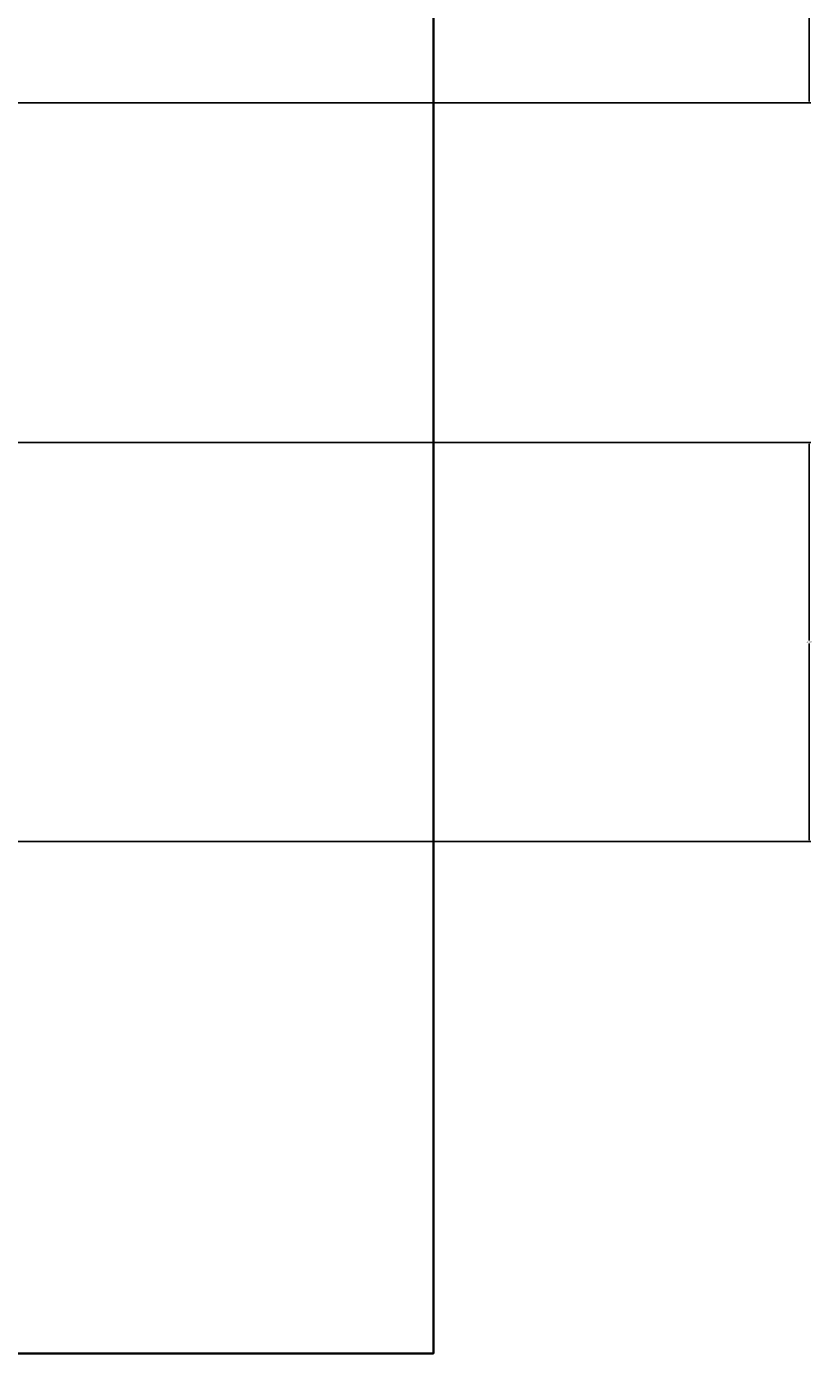
# Model space of a CAD drawing. Units: feet. Extents: x 2100 to 2836, y 2433 to 3396.
# Tile 5 of 12: x 2743 to 2836, y 2477 to 2634. Entities that reach past the tile are written whole.
import ezdxf

# ---------------------------------------------------------------- set-up
doc = ezdxf.new("R2010")
doc.units = ezdxf.units.FT
doc.layers.add('A-ANNO-DIMS', color=2, linetype='Continuous', lineweight=18)
doc.layers.add('A-ANNO-TTLB', color=7, linetype='Continuous', lineweight=35)
doc.styles.get("Standard").update_dxf_attribs({"font": 'arial.ttf'})
doc.dimstyles.get("Standard").update_dxf_attribs({"dimtxt": 0.18, "dimasz": 0.18, "dimexe": 0.18, "dimexo": 0.0625, "dimgap": 0.09, "dimtad": 0, "dimtih": 1, "dimtoh": 1, "dimdec": 4, "dimzin": 0, "dimdsep": 46, "dimtxsty": 'Standard', "dimcen": 0.09, "dimadec": 0, "dimazin": 0, "dimtfac": 1, "dimtdec": 4, "dimtofl": 0, "dimtmove": 0, "dimatfit": 3, "dimfxl": 1, "dimtolj": 1, "dimtzin": 0, "dimarcsym": 0})

# ---------------------------------------------------------------- blocks, each defined once
blk = doc.blocks.new('*D56')
at = {"layer": 'A-ANNO-DIMS', "color": 0, "lineweight": -2, "transparency": 16777216}
for p, q in [((2741.01, 2584.8), (2835.49, 2584.8)), ((2835.31, 2584.62), (2835.31, 2561.46)), ((2835.31, 2537.94), (2835.31, 2561.1)), ((2741.01, 2537.76), (2835.49, 2537.76))]:
    blk.add_line(p, q, dxfattribs=at)
at = {"layer": 'A-ANNO-DIMS', "color": 0, "transparency": 16777216}
for points in [[(2835.28, 2584.62), (2835.34, 2584.62), (2835.31, 2584.8)], [(2835.28, 2537.94), (2835.34, 2537.94), (2835.31, 2537.76)]]:
    blk.add_solid(points, dxfattribs=at)
at = {"layer": 'Defpoints', "color": 0, "transparency": 16777216}
for p in [(2740.95, 2584.8), (2835.31, 2584.8), (2740.95, 2537.76)]:
    blk.add_point(p, dxfattribs=at)
at = {"layer": 'A-ANNO-DIMS', "color": 0, "transparency": 16777216, "insert": (2835.31, 2561.28), "char_height": 0.18, "attachment_point": 5}
blk.add_mtext('\\A1;47.05', dxfattribs=at)
blk = doc.blocks.new('*D57')
at = {"layer": 'A-ANNO-DIMS', "color": 0, "lineweight": -2, "transparency": 16777216}
for p, q in [((2741.01, 2662.65), (2835.49, 2662.65)), ((2835.31, 2662.47), (2835.31, 2643.91)), ((2835.31, 2624.98), (2835.31, 2643.54)), ((2741.01, 2624.8), (2835.49, 2624.8))]:
    blk.add_line(p, q, dxfattribs=at)
at = {"layer": 'A-ANNO-DIMS', "color": 0, "transparency": 16777216}
for points in [[(2835.28, 2662.47), (2835.34, 2662.47), (2835.31, 2662.65)], [(2835.28, 2624.98), (2835.34, 2624.98), (2835.31, 2624.8)]]:
    blk.add_solid(points, dxfattribs=at)
at = {"layer": 'Defpoints', "color": 0, "transparency": 16777216}
for p in [(2740.95, 2662.65), (2835.31, 2662.65), (2740.95, 2624.8)]:
    blk.add_point(p, dxfattribs=at)
at = {"layer": 'A-ANNO-DIMS', "color": 0, "transparency": 16777216, "insert": (2835.31, 2643.73), "char_height": 0.18, "attachment_point": 5}
blk.add_mtext('\\A1;37.845', dxfattribs=at)

msp = doc.modelspace()

# ---------------------------------------------------------------- linework, layer by layer
at = {"layer": 'A-ANNO-TTLB'}
msp.add_lwpolyline([(2144.0848, 3351.6245), (2791.0561, 3351.6245), (2791.0561, 2477.4373), (2144.0848, 2477.4373)], close=True, dxfattribs=at)

# ---------------------------------------------------------------- dimensions: what is measured, and where the dimension line sits
at = {"layer": 'A-ANNO-DIMS'}
for base, p1, p2, override, picture, middle in [((2835.3061, 2662.6479), (2740.9476, 2624.8031), (2740.9476, 2662.6479), {"dimdec": 3, "dimlfac": 1, "dimrnd": 0, "dimzin": 0, "dimdsep": 46, "dimlunit": 2}, '*D57', (2835.3061, 2643.7255)), ((2835.3061, 2584.8031), (2740.9476, 2537.755), (2740.9476, 2584.8031), {"dimdec": 2, "dimlfac": 1, "dimrnd": 0, "dimzin": 0, "dimdsep": 46, "dimlunit": 2}, '*D56', (2835.3061, 2561.2791))]:
    dim = msp.add_linear_dim(base=base, p1=p1, p2=p2, angle=90, dimstyle='Standard', override=override, dxfattribs=at)
    dim.commit()
    dim.dimension.update_dxf_attribs({"geometry": picture, "text_midpoint": middle})

doc.saveas('drawing.dxf')
